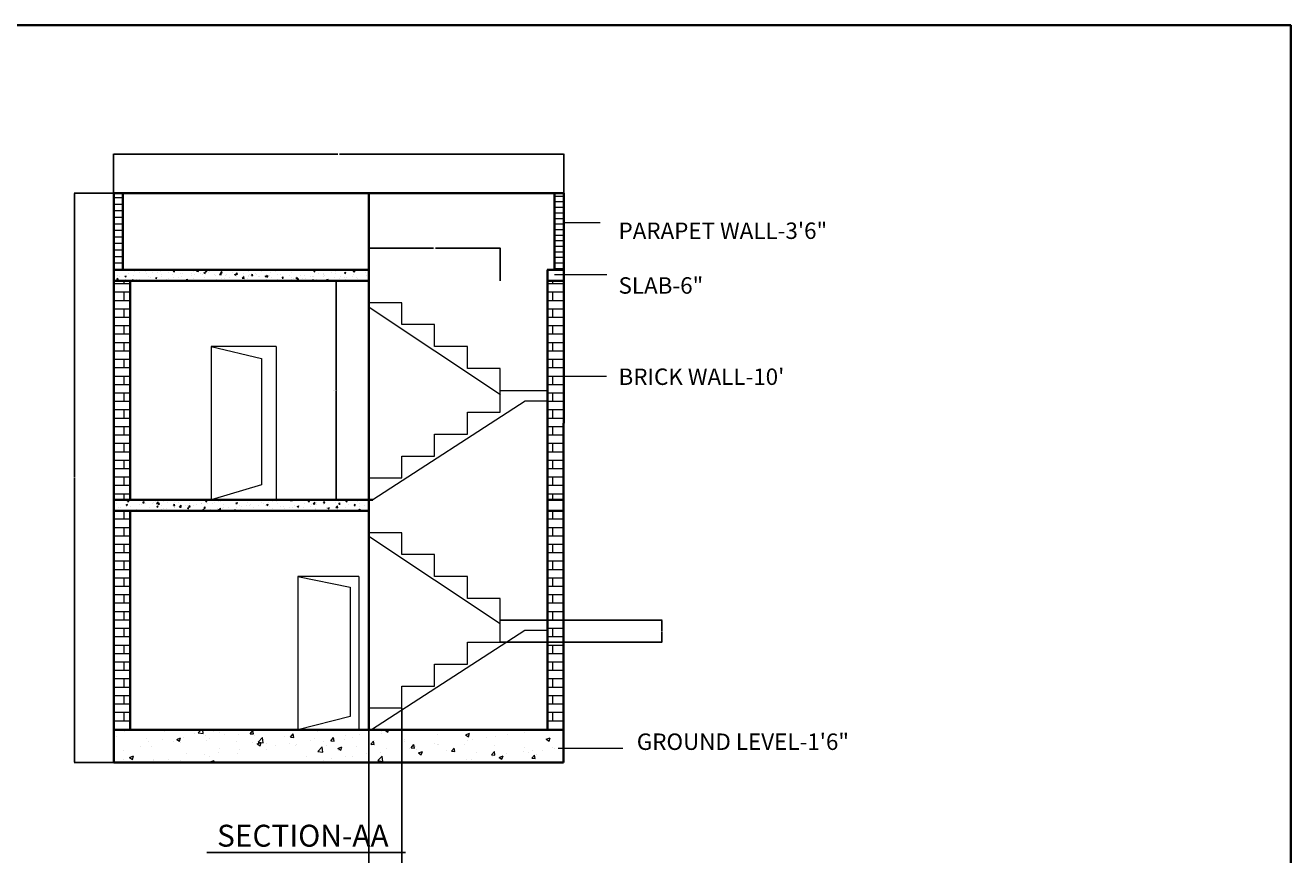
# Model space of a CAD drawing. Units: inches. Extents: x 1911 to 3278, y 2022 to 3108.
# Tile 13 of 13: x 2585 to 3278, y 2654 to 3108. Entities that reach past the tile are written whole.
import ezdxf

# ---------------------------------------------------------------- set-up
doc = ezdxf.new("R2010")
doc.units = ezdxf.units.IN
for name, color, linetype, lineweight in [('A-ANNO-DIMS', 2, 'Continuous', 18), ('A-ANNO-TEXT', 7, 'Continuous', 18), ('A-ANNO-TITL', 7, 'Continuous', 25), ('A-ANNO-TTLB', 7, 'Continuous', 35), ('A-DOOR', 4, 'Continuous', 18), ('A-FLOR-PATT', 252, 'Continuous', 13), ('A-FLOR-SLAB', 7, 'Continuous', 35), ('A-FLOR-STRS', 7, 'Continuous', 18), ('A-SECT', 7, 'Continuous', 35), ('A-WALL-PATT', 252, 'Continuous', 13)]:
    doc.layers.add(name, color=color, linetype=linetype, lineweight=lineweight)
doc.styles.get("Standard").update_dxf_attribs({"font": 'arial.ttf'})
doc.dimstyles.get("Standard").update_dxf_attribs({"dimtxt": 0.18, "dimasz": 0.18, "dimexe": 0.18, "dimexo": 0.0625, "dimgap": 0.09, "dimtad": 0, "dimtih": 1, "dimtoh": 1, "dimdec": 4, "dimzin": 0, "dimdsep": 46, "dimtxsty": 'Standard', "dimcen": 0.09, "dimadec": 0, "dimazin": 0, "dimtfac": 1, "dimtdec": 4, "dimtofl": 0, "dimtmove": 0, "dimatfit": 3, "dimfxl": 1, "dimtolj": 1, "dimtzin": 0, "dimarcsym": 0})

# ---------------------------------------------------------------- blocks, each defined once
blk = doc.blocks.new('STAIR-SECTION-TREAD-PROFILE')
for p, q in [((0, 108), (0, 120)), ((18, 108), (0, 108)), ((18, 96), (18, 108)), ((36, 96), (18, 96)), ((36, 84), (36, 96)), ((54, 84), (36, 84)), ((54, 72), (54, 84)), ((72, 72), (54, 72)), ((72, 60), (72, 72)), ((72, 48), (72, 60)), ((54, 36), (54, 48)), ((54, 48), (72, 48)), ((36, 24), (36, 36)), ((36, 36), (54, 36)), ((18, 12), (18, 24)), ((18, 24), (36, 24)), ((0, 0), (0, 12)), ((0, 12), (18, 12))]:
    blk.add_line(p, q)
blk = doc.blocks.new('*D64')
at = {"layer": 'A-ANNO-DIMS', "color": 0, "lineweight": -2, "transparency": 16777216}
for p, q in [((2773.14, 2968.03), (2755.02, 2968.03)), ((2755.2, 2967.85), (2755.2, 2908.21)), ((2755.2, 2848.21), (2755.2, 2907.84)), ((2773.14, 2848.03), (2755.02, 2848.03))]:
    blk.add_line(p, q, dxfattribs=at)
at = {"layer": 'A-ANNO-DIMS', "color": 0, "transparency": 16777216}
for points in [[(2755.17, 2967.85), (2755.23, 2967.85), (2755.2, 2968.03)], [(2755.17, 2848.21), (2755.23, 2848.21), (2755.2, 2848.03)]]:
    blk.add_solid(points, dxfattribs=at)
at = {"layer": 'Defpoints', "color": 0, "transparency": 16777216}
for p in [(2755.2, 2968.03), (2773.2, 2968.03), (2773.2, 2848.03)]:
    blk.add_point(p, dxfattribs=at)
at = {"layer": 'A-ANNO-DIMS', "color": 0, "transparency": 16777216, "insert": (2755.2, 2908.03), "char_height": 0.18, "attachment_point": 5}
blk.add_mtext('\\A1;FLIGHT PROFILE 120 TYP.', dxfattribs=at)
blk = doc.blocks.new('*D65')
at = {"layer": 'A-ANNO-DIMS', "color": 0, "lineweight": -2, "transparency": 16777216}
for p, q in [((2773.2, 2968.09), (2773.2, 2986.21)), ((2773.38, 2986.03), (2808.68, 2986.03)), ((2845.02, 2986.03), (2809.73, 2986.03)), ((2845.2, 2968.09), (2845.2, 2986.21))]:
    blk.add_line(p, q, dxfattribs=at)
at = {"layer": 'A-ANNO-DIMS', "color": 0, "transparency": 16777216}
for points in [[(2773.38, 2986.06), (2773.38, 2986), (2773.2, 2986.03)], [(2845.02, 2986.06), (2845.02, 2986), (2845.2, 2986.03)]]:
    blk.add_solid(points, dxfattribs=at)
at = {"layer": 'Defpoints', "color": 0, "transparency": 16777216}
for p in [(2845.2, 2986.03), (2773.2, 2968.03), (2845.2, 2968.03)]:
    blk.add_point(p, dxfattribs=at)
at = {"layer": 'A-ANNO-DIMS', "color": 0, "transparency": 16777216, "insert": (2809.2, 2986.03), "char_height": 0.18, "attachment_point": 5}
blk.add_mtext('\\A1;72 TYP.', dxfattribs=at)
blk = doc.blocks.new('*D97')
at = {"layer": 'A-ANNO-DIMS', "color": 0, "lineweight": -2, "transparency": 16777216}
for p, q in [((2633.35, 3016.09), (2633.35, 3037.61)), ((2633.53, 3037.43), (2756.21, 3037.43)), ((2879.82, 3037.43), (2757.14, 3037.43)), ((2880, 3016.09), (2880, 3037.61))]:
    blk.add_line(p, q, dxfattribs=at)
at = {"layer": 'A-ANNO-DIMS', "color": 0, "transparency": 16777216}
for points in [[(2633.53, 3037.46), (2633.53, 3037.4), (2633.35, 3037.43)], [(2879.82, 3037.46), (2879.82, 3037.4), (2880, 3037.43)]]:
    blk.add_solid(points, dxfattribs=at)
at = {"layer": 'Defpoints', "color": 0, "transparency": 16777216}
for p in [(2880, 3037.43), (2633.35, 3016.03), (2880, 3016.03)]:
    blk.add_point(p, dxfattribs=at)
at = {"layer": 'A-ANNO-DIMS', "color": 0, "transparency": 16777216, "insert": (2756.68, 3037.43), "char_height": 0.18, "attachment_point": 5}
blk.add_mtext('\\A1;246.65', dxfattribs=at)
blk = doc.blocks.new('*D98')
at = {"layer": 'A-ANNO-DIMS', "color": 0, "lineweight": -2, "transparency": 16777216}
for p, q in [((2633.29, 3016.03), (2611.77, 3016.03)), ((2611.95, 3015.85), (2611.95, 2860.21)), ((2611.95, 2704.21), (2611.95, 2859.85)), ((2633.29, 2704.03), (2611.77, 2704.03))]:
    blk.add_line(p, q, dxfattribs=at)
at = {"layer": 'A-ANNO-DIMS', "color": 0, "transparency": 16777216}
for points in [[(2611.92, 3015.85), (2611.98, 3015.85), (2611.95, 3016.03)], [(2611.92, 2704.21), (2611.98, 2704.21), (2611.95, 2704.03)]]:
    blk.add_solid(points, dxfattribs=at)
at = {"layer": 'Defpoints', "color": 0, "transparency": 16777216}
for p in [(2611.95, 3016.03), (2633.35, 3016.03), (2633.35, 2704.03)]:
    blk.add_point(p, dxfattribs=at)
at = {"layer": 'A-ANNO-DIMS', "color": 0, "transparency": 16777216, "insert": (2611.95, 2860.03), "char_height": 0.18, "attachment_point": 5}
blk.add_mtext('\\A1;312', dxfattribs=at)
blk = doc.blocks.new('*D99')
at = {"layer": 'A-ANNO-DIMS', "color": 0, "lineweight": -2, "transparency": 16777216}
for p, q in [((2773.2, 2733.96), (2773.2, 2633.15)), ((2791.2, 2733.96), (2791.2, 2633.15)), ((2773.38, 2633.33), (2781.99, 2633.33)), ((2791.02, 2633.33), (2782.42, 2633.33))]:
    blk.add_line(p, q, dxfattribs=at)
at = {"layer": 'A-ANNO-DIMS', "color": 0, "transparency": 16777216}
for points in [[(2773.38, 2633.36), (2773.38, 2633.3), (2773.2, 2633.33)], [(2791.02, 2633.36), (2791.02, 2633.3), (2791.2, 2633.33)]]:
    blk.add_solid(points, dxfattribs=at)
at = {"layer": 'Defpoints', "color": 0, "transparency": 16777216}
for p in [(2773.2, 2734.03), (2791.2, 2734.03), (2791.2, 2633.33)]:
    blk.add_point(p, dxfattribs=at)
at = {"layer": 'A-ANNO-DIMS', "color": 0, "transparency": 16777216, "insert": (2782.2, 2633.33), "char_height": 0.18, "attachment_point": 5}
blk.add_mtext('\\A1;18', dxfattribs=at)
blk = doc.blocks.new('*D100')
at = {"layer": 'A-ANNO-DIMS', "color": 0, "lineweight": -2, "transparency": 16777216}
for p, q in [((2845.27, 2782.03), (2933.87, 2782.03)), ((2933.69, 2781.85), (2933.69, 2776.21)), ((2933.69, 2770.21), (2933.69, 2775.85)), ((2845.27, 2770.03), (2933.87, 2770.03))]:
    blk.add_line(p, q, dxfattribs=at)
at = {"layer": 'A-ANNO-DIMS', "color": 0, "transparency": 16777216}
for points in [[(2933.66, 2781.85), (2933.72, 2781.85), (2933.69, 2782.03)], [(2933.66, 2770.21), (2933.72, 2770.21), (2933.69, 2770.03)]]:
    blk.add_solid(points, dxfattribs=at)
at = {"layer": 'Defpoints', "color": 0, "transparency": 16777216}
for p in [(2845.2, 2782.03), (2933.69, 2782.03), (2845.2, 2770.03)]:
    blk.add_point(p, dxfattribs=at)
at = {"layer": 'A-ANNO-DIMS', "color": 0, "transparency": 16777216, "insert": (2933.69, 2776.03), "char_height": 0.18, "attachment_point": 5}
blk.add_mtext('\\A1;12', dxfattribs=at)

msp = doc.modelspace()

# ---------------------------------------------------------------- hatches: boundary and pattern name
at = {"layer": 'A-FLOR-PATT'}
h = msp.add_hatch(dxfattribs=at)
h.set_pattern_fill('AR-CONC', color=256, scale=0.046, style=0)
h.paths.add_polyline_path([(2633.3539, 2968.0271), (2773.2046, 2968.0271), (2773.2046, 2974.0271), (2633.3539, 2974.0271)])
h = msp.add_hatch(dxfattribs=at)
h.set_pattern_fill('AR-CONC', color=256, scale=0.046, style=0)
h.paths.add_polyline_path([(2633.3539, 2842.0271), (2773.2046, 2842.0271), (2773.2046, 2848.0271), (2633.3539, 2848.0271)])
h = msp.add_hatch(dxfattribs=at)
h.set_pattern_fill('AR-CONC', color=256, scale=0.121, style=0)
h.paths.add_polyline_path([(2633.3539, 2704.0271), (2879.8539, 2704.0271), (2879.8539, 2722.0271), (2633.3539, 2722.0271)])
at = {"layer": 'A-WALL-PATT'}
h = msp.add_hatch(dxfattribs=at)
h.set_pattern_fill('LINE', color=256, scale=1.13, style=0)
h.paths.add_polyline_path([(2633.3539, 2974.0271), (2638.3231, 2974.0271), (2638.3231, 3016.0271), (2633.3539, 3016.0271)])
h = msp.add_hatch(dxfattribs=at)
h.set_pattern_fill('LINE', color=256, scale=0.96, style=0)
h.paths.add_polyline_path([(2874.8592, 2974.0271), (2880, 2974.0271), (2880, 3016.0271), (2874.8592, 3016.0271)])
h = msp.add_hatch(dxfattribs=at)
h.set_pattern_fill('AR-BRSTD', color=256, scale=0.068, style=0)
h.paths.add_polyline_path([(2633.3539, 2848.0271), (2642.3539, 2848.0271), (2642.3539, 2968.0271), (2633.3539, 2968.0271)])
h = msp.add_hatch(dxfattribs=at)
h.set_pattern_fill('AR-BRSTD', color=256, scale=0.068, style=0)
h.paths.add_polyline_path([(2871, 2848.0271), (2879.8539, 2848.0271), (2879.8539, 2890.0271), (2880, 2890.0271), (2880, 2968.0271), (2871, 2968.0271)])
h = msp.add_hatch(dxfattribs=at)
h.set_pattern_fill('AR-BRSTD', color=256, scale=0.068, style=0)
h.paths.add_polyline_path([(2633.3539, 2722.0271), (2642.3539, 2722.0271), (2642.3539, 2842.0271), (2633.3539, 2842.0271)])
h = msp.add_hatch(dxfattribs=at)
h.set_pattern_fill('AR-BRSTD', color=256, scale=0.068, style=0)
h.paths.add_polyline_path([(2871, 2722.0271), (2879.8539, 2722.0271), (2879.8539, 2842.0271), (2871, 2842.0271)])

# ---------------------------------------------------------------- linework, layer by layer
at = {"layer": 'A-ANNO-TEXT'}
for p, q in [((2880, 3000), (2900, 3000)), ((2874.8871, 2971.4874), (2903.6489, 2971.4874)), ((2880, 2915.769), (2903.3305, 2915.769)), ((2877.0075, 2711.933), (2912.2919, 2711.933))]:
    msp.add_line(p, q, dxfattribs=at)
at = {"layer": 'A-ANNO-TITL'}
msp.add_line((2684.3425, 2654.7258), (2793.3169, 2654.7258), dxfattribs=at)
at = {"layer": 'A-ANNO-TTLB'}
msp.add_lwpolyline([(1911.3875, 3108.0628), (3278.3142, 3108.0628), (3278.3142, 2021.7237), (1911.3875, 2021.7237)], close=True, dxfattribs=at)
at = {"layer": 'A-DOOR'}
for p, q in [((2686.7822, 2932.0271), (2686.7822, 2848.0271)), ((2722.4371, 2932.0271), (2686.7822, 2932.0271)), ((2686.7822, 2932.0271), (2714.3704, 2925.4822)), ((2722.4371, 2932.0271), (2722.4371, 2848.0271)), ((2714.3704, 2925.4822), (2714.3704, 2856.3156)), ((2714.3704, 2856.3156), (2686.7822, 2848.0271)), ((2734.3539, 2806.0271), (2734.3539, 2722.0271)), ((2767.757, 2806.0271), (2734.3539, 2806.0271)), ((2734.3539, 2806.0271), (2762.8933, 2800.1084)), ((2767.757, 2806.0271), (2767.757, 2722.0271)), ((2762.8933, 2800.1084), (2762.8933, 2729.3624)), ((2762.8933, 2729.3624), (2734.3539, 2722.0271))]:
    msp.add_line(p, q, dxfattribs=at)
at = {"layer": 'A-FLOR-SLAB'}
for p, q in [((2773.2046, 2974.0271), (2633.3539, 2974.0271)), ((2773.2046, 2968.0271), (2633.3539, 2968.0271)), ((2870.8539, 2974.0271), (2874.8592, 2974.0271)), ((2871, 2968.0271), (2871, 2974.0271)), ((2880, 2968.0271), (2871, 2968.0271)), ((2775.4418, 2848.0271), (2633.3539, 2848.0271)), ((2879.8539, 2848.0271), (2871, 2848.0271)), ((2773.2046, 2842.0271), (2633.3539, 2842.0271)), ((2879.8539, 2842.0271), (2871, 2842.0271)), ((2879.8539, 2722.0271), (2633.3539, 2722.0271)), ((2879.8539, 2704.0271), (2633.3539, 2704.0271))]:
    msp.add_line(p, q, dxfattribs=at)
at = {"layer": 'A-FLOR-STRS'}
for p, q in [((2773.3507, 2953.667), (2845.3507, 2905.7633)), ((2845.2046, 2908.0271), (2871, 2908.0271)), ((2858.7613, 2902.0636), (2775.4418, 2848.0271)), ((2871, 2902.0636), (2858.7613, 2902.0636)), ((2773.2046, 2842.0271), (2773.2046, 2848.0271)), ((2773.2046, 2828.0886), (2845.2046, 2780.1849)), ((2870.8539, 2782.0271), (2845.2046, 2782.0271)), ((2858.6152, 2776.4852), (2774.6456, 2722.0271)), ((2870.8539, 2776.4852), (2858.6152, 2776.4852)), ((2773.2046, 2722.0271), (2773.2046, 2731.0271))]:
    msp.add_line(p, q, dxfattribs=at)
at = {"layer": 'A-SECT'}
for p, q in [((2633.3539, 2890.0271), (2633.3539, 3016.0271)), ((2640, 3016.0271), (2633.3539, 3016.0271)), ((2638.3231, 2974.0271), (2638.3231, 3016.0271)), ((2773.2046, 3016.0271), (2640, 3016.0271)), ((2773.2046, 2722.0271), (2773.2046, 3016.0271)), ((2874.8592, 3016.0271), (2773.2046, 3016.0271)), ((2880, 3016.0271), (2874.8592, 3016.0271)), ((2874.8592, 2974.0271), (2874.8592, 3016.0271)), ((2880, 2890.0271), (2880, 3016.0271)), ((2642.3539, 2848.0271), (2642.3539, 2968.0271)), ((2871, 2968.0271), (2871, 2848.0271)), ((2880, 2974.0271), (2874.8592, 2974.0271)), ((2633.3539, 2890.0271), (2633.3539, 2704.0271)), ((2879.8539, 2890.0271), (2879.8539, 2704.0271)), ((2871, 2848.0271), (2871, 2722.0271)), ((2642.3539, 2842.0271), (2642.3539, 2722.0271))]:
    msp.add_line(p, q, dxfattribs=at)

# ---------------------------------------------------------------- block references
at = {"layer": 'A-FLOR-STRS'}
for p in [(2773.205, 2848.027), (2773.205, 2722.027)]:
    msp.add_blockref('STAIR-SECTION-TREAD-PROFILE', p, dxfattribs=at)

# ---------------------------------------------------------------- texts
at = {"layer": 'A-ANNO-TEXT', "char_height": 9, "attachment_point": 1}
for s, width, insert in [('PARAPET WALL-3\'6"', 140, (2910, 3000)), ('SLAB-6"', 110, (2910, 2970)), ("BRICK WALL-10'", 170, (2910, 2920)), ('GROUND LEVEL-1\'6"', 160, (2920, 2720))]:
    msp.add_mtext_dynamic_manual_height_columns(s, width=width, gutter_width=12.5, heights=[0], dxfattribs=dict(at, insert=insert))
at = {"layer": 'A-ANNO-TITL', "insert": (2690, 2670), "char_height": 12, "attachment_point": 1}
msp.add_mtext_dynamic_manual_height_columns('SECTION-AA', width=190, gutter_width=12.5, heights=[0], dxfattribs=at)

# ---------------------------------------------------------------- dimensions: what is measured, and where the dimension line sits
at = {"layer": 'A-ANNO-DIMS'}
for base, p1, p2, override, picture, middle in [((2880, 3037.4271), (2633.3539, 3016.0271), (2880, 3016.0271), {"dimdec": 2, "dimlfac": 1, "dimrnd": 0, "dimzin": 0, "dimdsep": 46, "dimlunit": 2}, '*D97', (2756.6769, 3037.4271)), ((2791.2046, 2633.3258), (2773.2046, 2734.0271), (2791.2046, 2734.0271), {"dimdec": 0, "dimlfac": 1, "dimrnd": 0, "dimzin": 0, "dimdsep": 46, "dimlunit": 2}, '*D99', (2782.2046, 2633.3258))]:
    dim = msp.add_linear_dim(base=base, p1=p1, p2=p2, dimstyle='Standard', override=override, dxfattribs=at)
    dim.commit()
    dim.dimension.update_dxf_attribs({"geometry": picture, "text_midpoint": middle})
for base, p1, p2, picture, middle in [((2611.9539, 3016.0271), (2633.3539, 2704.0271), (2633.3539, 3016.0271), '*D98', (2611.9539, 2860.0271)), ((2933.6919, 2782.0271), (2845.2046, 2770.0271), (2845.2046, 2782.0271), '*D100', (2933.6919, 2776.0271))]:
    dim = msp.add_linear_dim(base=base, p1=p1, p2=p2, angle=90, dimstyle='Standard', override={"dimdec": 0, "dimlfac": 1, "dimrnd": 0, "dimzin": 0, "dimdsep": 46, "dimlunit": 2}, dxfattribs=at)
    dim.commit()
    dim.dimension.update_dxf_attribs({"geometry": picture, "text_midpoint": middle})
dim = msp.add_linear_dim(base=(2845.2046, 2986.0271), p1=(2773.2046, 2968.0271), p2=(2845.2046, 2968.0271), text='<> TYP.', dimstyle='Standard', override={"dimdec": 0, "dimlfac": 1, "dimrnd": 0, "dimzin": 0, "dimdsep": 46, "dimlunit": 2}, dxfattribs=at)
dim.commit()
dim.dimension.update_dxf_attribs({"geometry": '*D65', "text_midpoint": (2809.2046, 2986.0271)})
dim = msp.add_linear_dim(base=(2755.2046, 2968.0271), p1=(2773.2046, 2848.0271), p2=(2773.2046, 2968.0271), angle=90, text='FLIGHT PROFILE <> TYP.', dimstyle='Standard', override={"dimdec": 0, "dimlfac": 1, "dimrnd": 0, "dimzin": 0, "dimdsep": 46, "dimlunit": 2}, dxfattribs=at)
dim.commit()
dim.dimension.update_dxf_attribs({"geometry": '*D64', "text_midpoint": (2755.2046, 2908.0271)})

doc.saveas('drawing.dxf')
